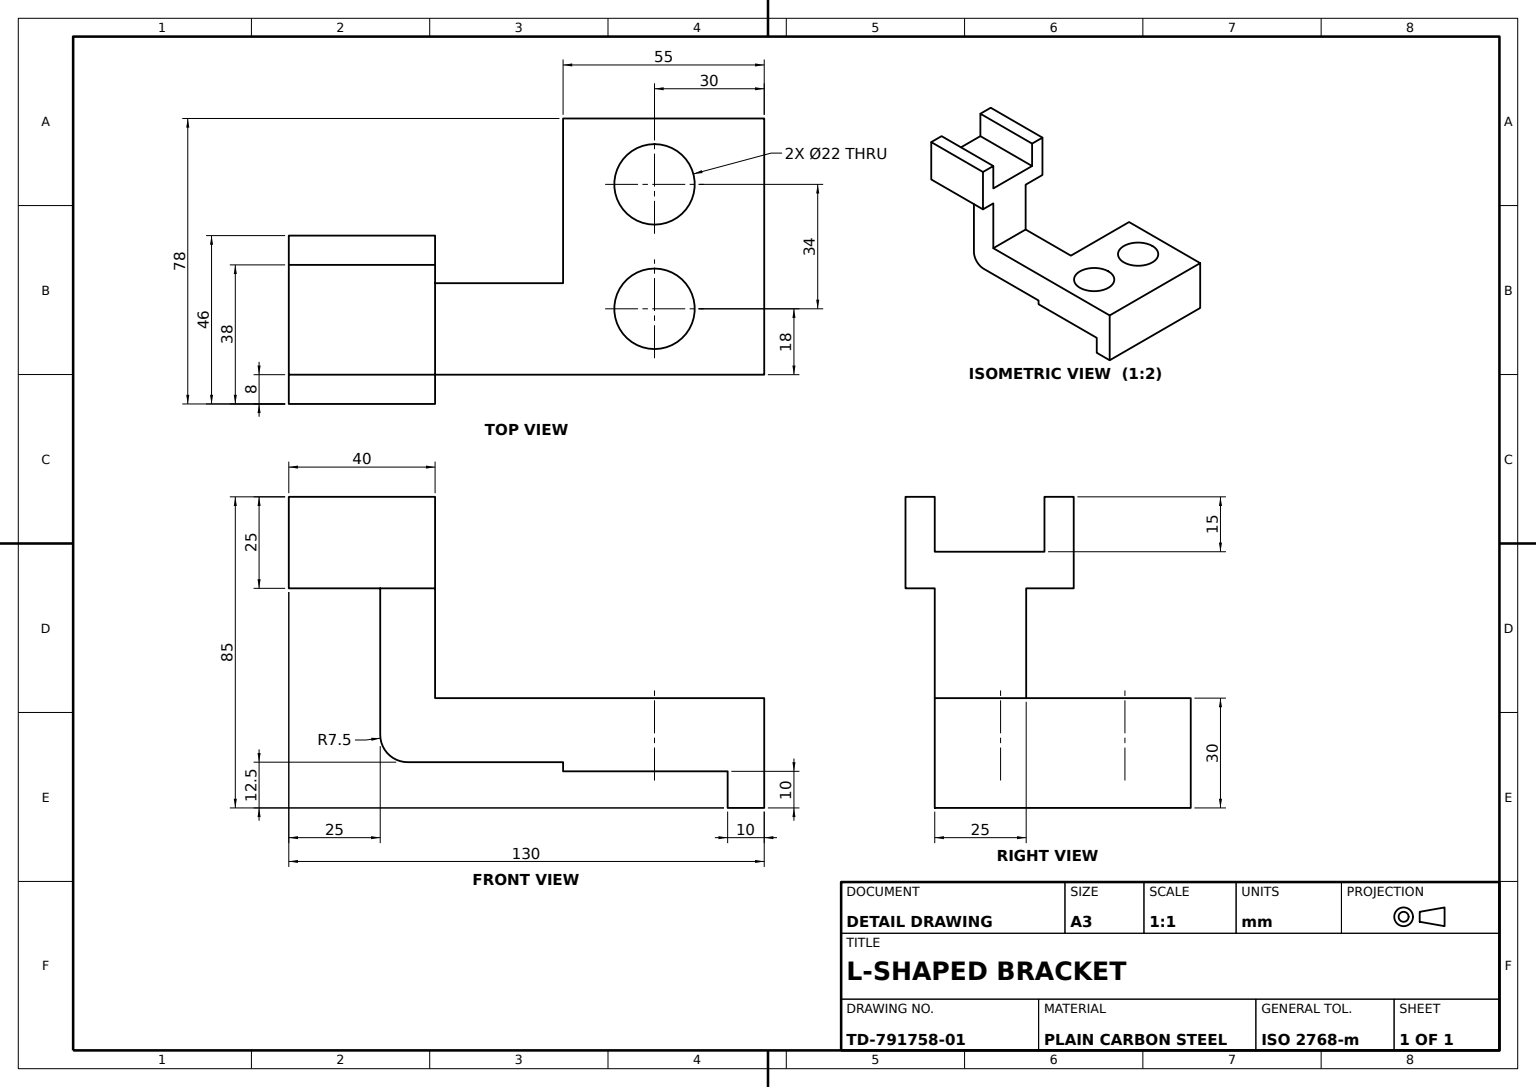
from build123d import *

# Parameters (mm, degrees)
BASE_BRACKET_DEPTH     = 70
UPRIGHT_POST_DEPTH     = 25
SLOTTED_HEAD_DEPTH     = 40
BASE_HOLES_SKETCH_R    = 11
BASE_HOLES_2X_22_DEPTH = 30


with BuildPart() as part:
    # Base Bracket Profile Sketch → Base Bracket (new body)
    with BuildSketch(Plane.XY):
        Polygon((0, 0), (45, 0), (45, -10), (55, -10), (55, 20), (0, 20), align=None)
    extrude(amount=BASE_BRACKET_DEPTH)

    # Upright Post Sketch → Upright Post (add)
    with BuildSketch(Plane.XY.offset(70)):
        with BuildLine():
            Line((-50, 50), (-50, 10))
            ThreePointArc((-50, 10), (-47.803300859, 4.696699141), (-42.5, 2.5))
            Line((-42.5, 2.5), (0, 2.5))
            Line((0, 2.5), (0, 20))
            Line((0, 20), (-35, 20))
            Line((-35, 20), (-35, 50))
            Line((-35, 50), (-50, 50))
        make_face()
    extrude(amount=-UPRIGHT_POST_DEPTH)

    # Slotted Head Profile Sketch → Slotted Head (add)
    with BuildSketch(Plane(origin=(-35, 0, 0), x_dir=(0, 0, -1), z_dir=(1, 0, 0))):
        Polygon((-70, 50), (-78, 50), (-78, 75), (-70, 75), (-70, 60), (-40, 60), (-40, 75), (-32, 75), (-32, 50), align=None)
    extrude(amount=-SLOTTED_HEAD_DEPTH)

    # Base Holes Sketch → Base Holes 2xØ22 (cut)
    with BuildSketch(Plane(origin=(0, 20, 0), x_dir=(1, 0, 0), z_dir=(0, 1, 0))):
        with Locations(Location((25, -18, 0), (0, 0, 270))):
            Circle(BASE_HOLES_SKETCH_R)
        with Locations(Location((25, -52, 0), (0, 0, 270))):
            Circle(BASE_HOLES_SKETCH_R)
    extrude(amount=-BASE_HOLES_2X_22_DEPTH, mode=Mode.SUBTRACT)


solid = part.part
